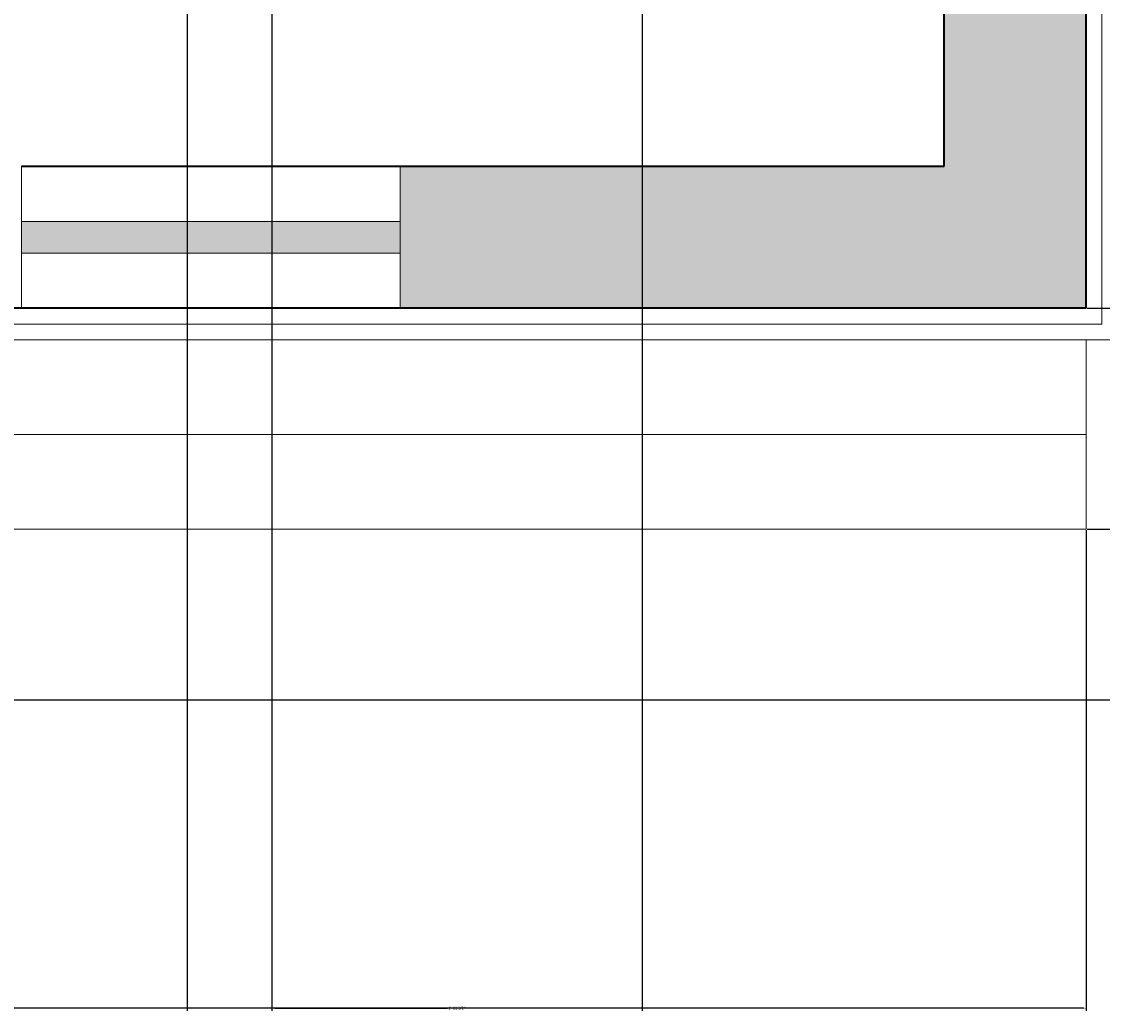
# Model space of a CAD drawing. Units: inches. Extents: x 311 to 815, y -527 to 136.
# Tile 10 of 21: x 655 to 723, y -527 to -464. Entities that reach past the tile are written whole.
import ezdxf

# ---------------------------------------------------------------- set-up
doc = ezdxf.new("R2010")
doc.units = ezdxf.units.IN
doc.header["$MEASUREMENT"] = 0
for name, color, linetype, lineweight in [('A-ANNO-DIMS', 1, 'Continuous', 18), ('A-ANNO-TTLB', 1, 'Continuous', 25), ('A-FLOR-EDGE', 1, 'Continuous', 18), ('A-FLOR-STRS', 1, 'Continuous', 18), ('A-GLAZ-PATT', 5, 'Continuous', 13), ('A-WALL-PATT', 242, 'Continuous', 13), ('wall', 1, 'Continuous', 35), ('win', 5, 'Continuous', 18)]:
    doc.layers.add(name, color=color, linetype=linetype, lineweight=lineweight)
doc.styles.get("Standard").update_dxf_attribs({"font": 'arial.ttf'})
doc.dimstyles.get("Standard").update_dxf_attribs({"dimtxt": 0.18, "dimasz": 0.18, "dimexe": 0.18, "dimexo": 0.0625, "dimgap": 0.09, "dimtad": 0, "dimtih": 1, "dimtoh": 1, "dimdec": 1, "dimzin": 0, "dimdsep": 46, "dimlunit": 4, "dimtxsty": 'Standard', "dimcen": 0.09, "dimadec": 0, "dimazin": 0, "dimtfac": 1, "dimtdec": 1, "dimtofl": 0, "dimtmove": 0, "dimatfit": 3, "dimfxl": 1, "dimtolj": 1, "dimtzin": 0, "dimarcsym": 0})

# ---------------------------------------------------------------- blocks, each defined once
blk = doc.blocks.new('WIN-24IN')
for p, q in [((9, 24), (0, 24)), ((3.5, 0), (3.5, 24)), ((5.5, 0), (5.5, 24)), ((9, 0), (0, 0))]:
    blk.add_line(p, q)
blk = doc.blocks.new('*D23')
at = {"layer": 'A-ANNO-DIMS', "color": 0, "lineweight": -2, "transparency": 16777216}
for p, q in [((548.323, -496.19), (548.323, -526.658)), ((722.331, -496.19), (722.331, -526.658)), ((548.503, -526.478), (634.936, -526.478)), ((722.151, -526.478), (635.718, -526.478))]:
    blk.add_line(p, q, dxfattribs=at)
at = {"layer": 'A-ANNO-DIMS', "color": 0, "transparency": 16777216}
for points in [[(548.503, -526.448), (548.503, -526.508), (548.323, -526.478)], [(722.151, -526.448), (722.151, -526.508), (722.331, -526.478)]]:
    blk.add_solid(points, dxfattribs=at)
at = {"layer": 'Defpoints', "color": 0, "transparency": 16777216}
for p in [(548.323, -496.128), (722.331, -496.128), (722.331, -526.478)]:
    blk.add_point(p, dxfattribs=at)
at = {"layer": 'A-ANNO-DIMS', "color": 0, "transparency": 16777216, "insert": (635.327, -526.478), "char_height": 0.18, "attachment_point": 5}
blk.add_mtext('\\A1;14\'-6"', dxfattribs=at)
blk = doc.blocks.new('*D24')
at = {"layer": 'A-ANNO-DIMS', "color": 0, "lineweight": -2, "transparency": 16777216}
for p, q in [((722.385, -482.128), (754.853, -482.128)), ((754.673, -482.308), (754.673, -488.947)), ((754.673, -495.948), (754.673, -489.308)), ((722.394, -496.128), (754.853, -496.128))]:
    blk.add_line(p, q, dxfattribs=at)
at = {"layer": 'A-ANNO-DIMS', "color": 0, "transparency": 16777216}
for points in [[(754.643, -482.308), (754.703, -482.308), (754.673, -482.128)], [(754.643, -495.948), (754.703, -495.948), (754.673, -496.128)]]:
    blk.add_solid(points, dxfattribs=at)
at = {"layer": 'Defpoints', "color": 0, "transparency": 16777216}
for p in [(722.323, -482.128), (722.331, -496.128), (754.673, -496.128)]:
    blk.add_point(p, dxfattribs=at)
at = {"layer": 'A-ANNO-DIMS', "color": 0, "transparency": 16777216, "insert": (754.673, -489.128), "char_height": 0.18, "attachment_point": 5}
blk.add_mtext('\\A1;1\'-2"', dxfattribs=at)
blk = doc.blocks.new('*D30')
at = {"layer": 'A-ANNO-DIMS', "color": 0, "lineweight": -2, "transparency": 16777216}
for p, q in [((722.385, -445.128), (754.853, -445.128)), ((754.673, -445.308), (754.673, -463.446)), ((754.673, -481.948), (754.673, -463.81)), ((722.385, -482.128), (754.853, -482.128))]:
    blk.add_line(p, q, dxfattribs=at)
at = {"layer": 'A-ANNO-DIMS', "color": 0, "transparency": 16777216}
for points in [[(754.643, -445.308), (754.703, -445.308), (754.673, -445.128)], [(754.643, -481.948), (754.703, -481.948), (754.673, -482.128)]]:
    blk.add_solid(points, dxfattribs=at)
at = {"layer": 'Defpoints', "color": 0, "transparency": 16777216}
for p in [(722.323, -445.128), (754.673, -445.128), (722.323, -482.128)]:
    blk.add_point(p, dxfattribs=at)
at = {"layer": 'A-ANNO-DIMS', "color": 0, "transparency": 16777216, "insert": (754.673, -463.628), "char_height": 0.18, "attachment_point": 5}
blk.add_mtext('\\A1;3\'-1"', dxfattribs=at)
blk = doc.blocks.new('*D31')
at = {"layer": 'A-ANNO-DIMS', "color": 0, "lineweight": -2, "transparency": 16777216}
for p, q in [((670.696, -191.608), (670.696, -526.658)), ((694.164, -191.608), (694.164, -526.658)), ((670.876, -526.478), (681.83, -526.478)), ((693.984, -526.478), (683.03, -526.478))]:
    blk.add_line(p, q, dxfattribs=at)
at = {"layer": 'A-ANNO-DIMS', "color": 0, "transparency": 16777216}
for points in [[(670.876, -526.448), (670.876, -526.508), (670.696, -526.478)], [(693.984, -526.448), (693.984, -526.508), (694.164, -526.478)]]:
    blk.add_solid(points, dxfattribs=at)
at = {"layer": 'Defpoints', "color": 0, "transparency": 16777216}
for p in [(670.696, -191.545), (694.164, -191.545), (694.164, -526.478)]:
    blk.add_point(p, dxfattribs=at)
at = {"layer": 'A-ANNO-DIMS', "color": 0, "transparency": 16777216, "insert": (682.43, -526.478), "char_height": 0.18, "attachment_point": 5}
blk.add_mtext('\\A1;1\'-11 1/2"', dxfattribs=at)
blk = doc.blocks.new('*D37')
at = {"layer": 'A-ANNO-DIMS', "color": 0, "lineweight": -2, "transparency": 16777216}
for p, q in [((633.323, -348.19), (633.323, -526.658)), ((665.323, -348.19), (665.323, -526.658)), ((633.503, -526.478), (648.992, -526.478)), ((665.143, -526.478), (649.654, -526.478))]:
    blk.add_line(p, q, dxfattribs=at)
at = {"layer": 'A-ANNO-DIMS', "color": 0, "transparency": 16777216}
for points in [[(633.503, -526.448), (633.503, -526.508), (633.323, -526.478)], [(665.143, -526.448), (665.143, -526.508), (665.323, -526.478)]]:
    blk.add_solid(points, dxfattribs=at)
at = {"layer": 'Defpoints', "color": 0, "transparency": 16777216}
for p in [(633.323, -348.128), (665.323, -348.128), (665.323, -526.478)]:
    blk.add_point(p, dxfattribs=at)
at = {"layer": 'A-ANNO-DIMS', "color": 0, "transparency": 16777216, "insert": (649.323, -526.478), "char_height": 0.18, "attachment_point": 5}
blk.add_mtext('\\A1;2\'-8"', dxfattribs=at)

msp = doc.modelspace()

# ---------------------------------------------------------------- hatches: boundary and pattern name
at = {"layer": 'A-GLAZ-PATT'}
h = msp.add_hatch(color=256, dxfattribs=at)
h.dxf.hatch_style = 1
h.paths.add_polyline_path([(415.823, -202.128), (413.823, -202.128), (413.823, -262.128), (415.823, -262.128)])
h.paths.add_polyline_path([(415.823, -390.84), (413.823, -390.84), (413.823, -450.84), (415.823, -450.84)])
h.paths.add_polyline_path([(415.823, -311.568), (413.823, -311.568), (413.823, -335.568), (415.823, -335.568)])
h.paths.add_polyline_path([(509.323, -476.628), (449.323, -476.628), (449.323, -478.628), (509.323, -478.628)])
h.paths.add_polyline_path([(606.823, -476.628), (582.823, -476.628), (582.823, -478.628), (606.823, -478.628)])
h.paths.add_polyline_path([(678.823, -476.628), (654.823, -476.628), (654.823, -478.628), (678.823, -478.628)])
h.paths.add_polyline_path([(718.823, -385.128), (716.823, -385.128), (716.823, -445.128), (718.823, -445.128)])
h.paths.add_polyline_path([(718.823, -262.628), (716.823, -262.628), (716.823, -322.628), (718.823, -322.628)])
h.paths.add_polyline_path([(718.823, -140.128), (716.823, -140.128), (716.823, -200.128), (718.823, -200.128)])
h.paths.add_polyline_path([(718.823, -18.128), (716.823, -18.128), (716.823, -42.128), (718.823, -42.128)])
h.paths.add_polyline_path([(686.823, 18.372), (626.823, 18.372), (626.823, 16.372), (686.823, 16.372)])
h.paths.add_polyline_path([(581.823, 18.372), (557.823, 18.372), (557.823, 16.372), (581.823, 16.372)])
h.paths.add_polyline_path([(509.323, 18.372), (449.323, 18.372), (449.323, 16.372), (509.323, 16.372)])
at = {"layer": 'A-WALL-PATT'}
h = msp.add_hatch(color=256, dxfattribs=at)
h.dxf.hatch_style = 1
h.paths.add_polyline_path([(557.823, 21.872), (509.323, 21.872), (509.323, 12.872), (539.323, 12.872), (539.323, -112.128), (548.323, -112.128), (548.323, -58.628), (557.823, -58.628), (557.823, -49.628), (548.323, -49.628), (548.323, 12.872), (557.823, 12.872)])
h.paths.add_polyline_path([(449.323, 21.872), (410.323, 21.872), (410.323, -15.128), (419.323, -15.128), (419.323, 12.872), (449.323, 12.872)])
h.paths.add_polyline_path([(626.823, 21.872), (581.823, 21.872), (581.823, 12.872), (591.323, 12.872), (591.323, -49.628), (581.823, -49.628), (581.823, -58.628), (591.323, -58.628), (591.323, -112.128), (600.323, -112.128), (600.323, 12.872), (626.823, 12.872)])
h.paths.add_polyline_path([(722.323, 21.872), (686.823, 21.872), (686.823, 12.872), (713.323, 12.872), (713.323, -18.128), (722.323, -18.128)])
h.paths.add_polyline_path([(722.323, -42.128), (713.323, -42.128), (713.323, -73.128), (722.323, -73.128)])
h.paths.add_polyline_path([(501.323, -103.128), (419.323, -103.128), (419.323, -75.128), (410.323, -75.128), (410.323, -126.628), (419.323, -126.628), (419.323, -112.128), (492.323, -112.128), (492.323, -143.128), (501.323, -143.128)])
h.paths.add_polyline_path([(548.323, -165.128), (419.323, -165.128), (419.323, -150.628), (410.323, -150.628), (410.323, -202.128), (419.323, -202.128), (419.323, -174.128), (548.323, -174.128)])
h.paths.add_polyline_path([(722.323, -103.128), (636.323, -103.128), (636.323, -112.128), (713.323, -112.128), (713.323, -140.128), (722.323, -140.128)])
h.paths.add_polyline_path([(548.323, -210.128), (539.323, -210.128), (539.323, -290.128), (419.323, -290.128), (419.323, -262.128), (410.323, -262.128), (410.323, -311.568), (419.323, -311.568), (419.323, -299.128), (469.323, -299.128), (469.323, -348.128), (443.323, -348.128), (443.323, -357.128), (478.323, -357.128), (478.323, -299.128), (548.323, -299.128)])
h.paths.add_polyline_path([(722.323, -200.128), (713.323, -200.128), (713.323, -228.128), (609.323, -228.128), (609.323, -237.128), (713.323, -237.128), (713.323, -262.628), (722.323, -262.628)])
h.paths.add_polyline_path([(722.323, -322.628), (713.323, -322.628), (713.323, -348.128), (633.323, -348.128), (633.323, -357.128), (713.323, -357.128), (713.323, -385.128), (722.323, -385.128)])
h.paths.add_polyline_path([(419.323, -335.568), (410.323, -335.568), (410.323, -390.84), (419.323, -390.84)])
h.paths.add_polyline_path([(419.323, -450.84), (410.323, -450.84), (410.323, -482.128), (449.323, -482.128), (449.323, -473.128), (419.323, -473.128)])
h.paths.add_polyline_path([(582.823, -473.128), (548.323, -473.128), (548.323, -348.128), (539.323, -348.128), (539.323, -473.128), (509.323, -473.128), (509.323, -482.128), (582.823, -482.128)])
h.paths.add_polyline_path([(722.323, -445.128), (713.323, -445.128), (713.323, -473.128), (678.823, -473.128), (678.823, -482.128), (722.323, -482.128)])

# ---------------------------------------------------------------- linework, layer by layer
at = {"layer": 'A-ANNO-TTLB'}
msp.add_lwpolyline([(310.674, 136.008), (815.429, 136.008), (815.429, -506.965), (310.674, -506.965)], close=True, dxfattribs=at)
at = {"layer": 'A-FLOR-EDGE'}
for p, q in [((723.323, -483.128), (723.323, 22.872)), ((723.323, -483.128), (409.323, -483.128)), ((724.323, -484.128), (408.323, -484.128))]:
    msp.add_line(p, q, dxfattribs=at)
at = {"layer": 'A-FLOR-STRS'}
for p, q in [((722.331, -484.128), (722.331, -496.128)), ((548.323, -490.128), (722.331, -490.128)), ((722.331, -496.128), (548.323, -496.128))]:
    msp.add_line(p, q, dxfattribs=at)
at = {"layer": 'wall'}
for p, q in [((722.323, -482.128), (722.323, -103.128)), ((713.323, -473.128), (713.323, -357.128)), ((654.823, -473.128), (713.323, -473.128)), ((722.323, -482.128), (410.323, -482.128))]:
    msp.add_line(p, q, dxfattribs=at)

# ---------------------------------------------------------------- block references
at = {"layer": 'win', "rotation": 90.00000000000003}
msp.add_blockref('WIN-24IN', (678.823, -482.128), dxfattribs=at)

# ---------------------------------------------------------------- dimensions: what is measured, and where the dimension line sits
at = {"layer": 'A-ANNO-DIMS'}
for base, p1, p2, picture, middle in [((694.164, -526.478), (670.696, -191.545), (694.164, -191.545), '*D31', (682.43, -526.478)), ((665.323, -526.478), (633.323, -348.128), (665.323, -348.128), '*D37', (649.323, -526.478)), ((722.331, -526.478), (548.323, -496.128), (722.331, -496.128), '*D23', (635.327, -526.478))]:
    dim = msp.add_linear_dim(base=base, p1=p1, p2=p2, dimstyle='Standard', override={"dimdec": 1, "dimlfac": 1, "dimrnd": 0, "dimzin": 1, "dimdsep": 46, "dimlunit": 4, "dimfrac": 2}, dxfattribs=at)
    dim.commit()
    dim.dimension.update_dxf_attribs({"geometry": picture, "text_midpoint": middle})
for base, p2, picture, middle in [((754.673, -445.128), (722.323, -445.128), '*D30', (754.673, -463.628)), ((754.673, -496.128), (722.331, -496.128), '*D24', (754.673, -489.128))]:
    dim = msp.add_linear_dim(base=base, p1=(722.323, -482.128), p2=p2, angle=90, dimstyle='Standard', override={"dimdec": 1, "dimlfac": 1, "dimrnd": 0, "dimzin": 1, "dimdsep": 46, "dimlunit": 4, "dimfrac": 2}, dxfattribs=at)
    dim.commit()
    dim.dimension.update_dxf_attribs({"geometry": picture, "text_midpoint": middle})

doc.saveas('drawing.dxf')
